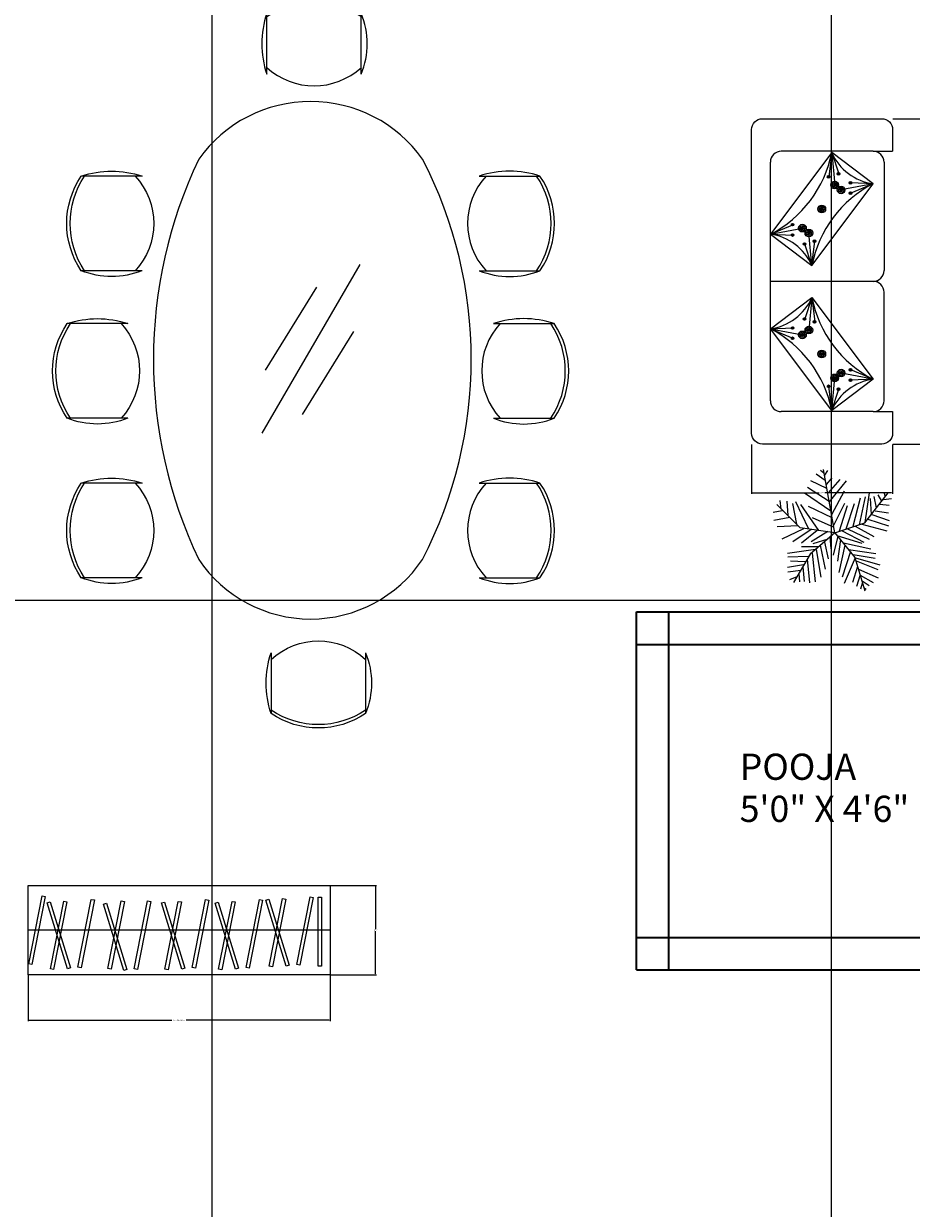
# Model space of a CAD drawing. Units: inches. Extents: x -61 to 1599, y -1316 to 257.
# Tile 196 of 204: x 1233 to 1396, y -279 to -61. Entities that reach past the tile are written whole.
import ezdxf

# ---------------------------------------------------------------- set-up
doc = ezdxf.new("R2010")
doc.units = ezdxf.units.IN
doc.header["$MEASUREMENT"] = 0
for name, color, linetype, lineweight in [('A-ANNO-DIMS', 2, 'Continuous', 18), ('A-AREA-IDEN', 1, 'Continuous', 18), ('A-FLOR-CASE', 8, 'Continuous', 18), ('FURNITURE', 83, 'Continuous', 18), ('WALLS', 4, 'Continuous', 35)]:
    doc.layers.add(name, color=color, linetype=linetype, lineweight=lineweight)
doc.layers.add('FUR', color=83, linetype='Continuous')
doc.styles.get("Standard").update_dxf_attribs({"font": 'arial.ttf'})
doc.dimstyles.get("Standard").update_dxf_attribs({"dimtxt": 0.18, "dimasz": 0.18, "dimexe": 0.18, "dimexo": 0.0625, "dimgap": 0.09, "dimtad": 0, "dimtih": 1, "dimtoh": 1, "dimdec": 0, "dimzin": 0, "dimdsep": 46, "dimlunit": 3, "dimtxsty": 'Standard', "dimcen": 0.09, "dimadec": 0, "dimazin": 0, "dimtfac": 1, "dimtdec": 0, "dimtofl": 0, "dimtmove": 0, "dimatfit": 3, "dimfxl": 1, "dimtolj": 1, "dimtzin": 0, "dimarcsym": 0})

# ---------------------------------------------------------------- blocks, each defined once
blk = doc.blocks.new('*U264')
for p, q in [((-10.186, 53.64), (-13.084, 55.962)), ((0, 0), (-10.5, 57)), ((-9.099, 51.782), (-6.563, 55.962)), ((-7.288, 39.707), (-21.778, 46.673)), ((-8.737, 47.138), (-17.069, 52.711)), ((-7.65, 43.423), (-2.578, 49.46)), ((-5.839, 35.992), (4.667, 48.067)), ((-5.114, 27.632), (10.463, 46.673)), ((-3.665, 19.273), (-27.574, 35.527)), ((-5.114, 28.097), (-24.676, 40.636)), ((-2.941, 16.486), (8.652, 37.85)), ((22.055, 7.198), (27.489, 32.277)), ((27, 9), (48, 36)), ((27.127, 9.056), (31.112, 35.992)), ((35.096, 32.741), (37.27, 22.524)), ((38.719, 34.134), (41.979, 28.561)), ((44.153, 36.456), (45.239, 32.741)), ((-31.5, 4.5), (-52.5, 25.5)), ((-48.585, 21.131), (-49.309, 29.026)), ((-43.513, 28.561), (-42.427, 15.558)), ((-38.442, 26.239), (-34.819, 7.663)), ((-35.544, 28.097), (-24.314, 3.947)), ((-14.533, 2.09), (-30.834, 25.31)), ((-24.314, 23.917), (-2.941, 13.7)), ((-1.129, 6.734), (9.014, 26.704)), ((3.942, 1.625), (11.187, 24.381)), ((10.101, 3.483), (17.708, 26.239)), ((16.259, 5.805), (23.142, 31.348)), ((31.836, 30.883), (32.561, 16.486)), ((40.53, 25.775), (48.862, 24.846)), ((43.791, 29.954), (51.036, 30.883)), ((-47.498, 19.737), (-55.83, 18.344)), ((-40.615, 13.7), (-55.105, 10.913)), ((-20.691, 13.7), (-1.129, 4.876)), ((29.662, 12.307), (48.137, 6.269)), ((33.285, 16.486), (48.862, 10.913)), ((36.183, 19.737), (48.137, 17.88)), ((-33.37, 6.269), (-52.207, 5.34)), ((-28.299, 3.483), (-47.86, -5.805)), ((-21.416, 3.018), (-38.079, -8.128)), ((0, 0), (-31.5, 4.5)), ((-15.982, 2.09), (-30.11, -9.521)), ((0, 0), (-22.5, -19.5)), ((-6.563, 1.161), (-21.416, -8.128)), ((0, 0), (27, 9)), ((0, 0), (18, -22.5)), ((6.478, 1.625), (26.04, -8.592)), ((11.187, 3.483), (30.749, -5.805)), ((18.07, 5.805), (35.096, -3.483)), ((24.229, 7.663), (46.688, 1.625)), ((-6.563, -5.805), (-19.967, -9.985)), ((-9.461, -8.592), (-6.201, -23.453)), ((-4.752, -3.483), (-3.665, -14.629)), ((2.493, -3.019), (-1.491, -20.202)), ((1.769, -2.555), (24.229, -9.521)), ((5.029, -6.27), (2.131, -25.775)), ((7.565, -9.056), (32.198, -14.629)), ((-17.431, -15.094), (-42.789, -18.809)), ((-22.5, -19.5), (-37.5, -45)), ((-15.257, -12.772), (-30.11, -12.772)), ((-20.691, -18.345), (-17.793, -44.352)), ((-17.069, -15.094), (-12.721, -40.172)), ((-13.446, -11.378), (-8.737, -32.741)), ((9.014, -11.378), (3.58, -35.992)), ((14.085, -16.951), (6.478, -40.172)), ((12.274, -15.094), (36.907, -18.809)), ((16.259, -19.738), (36.183, -22.989)), ((-28.299, -29.026), (-42.789, -31.348)), ((-24.314, -21.596), (-42.427, -22.06)), ((-26.849, -26.24), (-40.253, -25.775)), ((-29.023, -30.884), (-27.936, -43.887)), ((-25.038, -23.918), (-22.865, -45.281)), ((18.07, -22.524), (8.289, -45.745)), ((20.244, -30.419), (15.897, -44.816)), ((18, -22.5), (27, -52.5)), ((18.433, -22.524), (40.53, -29.026)), ((19.157, -25.311), (38.719, -33.206)), ((-30.834, -34.135), (-42.427, -35.528)), ((-34.457, -39.708), (-40.978, -42.494)), ((-32.646, -36.921), (-31.921, -44.352)), ((22.78, -37.85), (19.519, -48.532)), ((21.331, -32.741), (39.081, -40.636)), ((22.78, -38.314), (34.372, -44.816)), ((24.591, -45.745), (23.142, -50.854)), ((24.591, -43.423), (30.749, -47.603)), ((26.764, -49.925), (28.213, -50.854))]:
    blk.add_line(p, q)
blk = doc.blocks.new('DINING-TABLE-OVAL')
for p, q in [((20.06, 34.26), (38.12, 65.35)), ((20.69, 45.86), (30.12, 61.18)), ((27.51, 37.68), (36.94, 53.01))]:
    blk.add_line(p, q)
for centre, radius, start, end in [((28.99, 70.07), 25.36, 35.5172, 144.4828), ((85.79, 47.89), 85.79, 154.5151, 205.4849), ((-21.85, 47.89), 80.45, 332.689, 27.311), ((28.99, 24.89), 24.89, 213.9753, 326.0247)]:
    blk.add_arc(centre, radius, start, end)
blk = doc.blocks.new('DINING-CHAIR')
for p, q in [((0.9, 2.16), (0.9, 13.35)), ((18.35, 2.16), (18.35, 13.35))]:
    blk.add_line(p, q)
for centre, radius, start, end in [((9.63, 0.52), 15.52, 55.8098, 124.1902), ((9.63, -0.1), 15.52, 55.8098, 124.1902), ((17.78, 7.76), 17.78, 161.6455, 198.3545), ((4.51, 7.76), 14.92, 337.9646, 22.0354), ((9.63, 12.87), 12.87, 227.332, 312.668)]:
    blk.add_arc(centre, radius, start, end)
blk = doc.blocks.new('WARDROBE-HANGING-2')
blk.add_line((55.7, 8.23), (0, 8.23))
for points in [[(55.7, 16.46), (55.7, 0), (0, 0), (0, 16.46)], [(0.12, 2.03), (2.58, 14.54), (3.16, 14.43), (0.7, 1.92)], [(7.24, 1.1), (3.5, 13.29), (4.06, 13.46), (7.8, 1.28)], [(4.13, 1.08), (6.59, 13.59), (7.17, 13.48), (4.71, 0.97)], [(9.19, 1.4), (11.65, 13.91), (12.23, 13.8), (9.77, 1.29)], [(17.64, 0.82), (13.9, 13), (14.46, 13.18), (18.2, 0.99)], [(14.73, 1.14), (17.19, 13.65), (17.77, 13.54), (15.31, 1.03)], [(19.59, 1.12), (22.05, 13.62), (22.63, 13.51), (20.17, 1)], [(28.34, 1.05), (24.59, 13.24), (25.16, 13.41), (28.9, 1.22)], [(25.23, 1.03), (27.69, 13.54), (28.27, 13.43), (25.81, 0.92)], [(30.28, 1.35), (32.74, 13.86), (33.32, 13.75), (30.86, 1.24)], [(38.26, 1.05), (34.51, 13.23), (35.08, 13.41), (38.82, 1.22)], [(35.15, 1.03), (37.61, 13.54), (38.19, 13.42), (35.73, 0.92)], [(40.2, 1.35), (42.66, 13.86), (43.24, 13.74), (40.78, 1.23)], [(47.6, 1.58), (43.86, 13.76), (44.42, 13.94), (48.16, 1.75)], [(44.49, 1.56), (46.95, 14.07), (47.53, 13.95), (45.07, 1.45)], [(49.55, 1.88), (52.01, 14.39), (52.59, 14.27), (50.13, 1.77)], [(54.1, 14.33), (54.1, 1.58), (53.51, 1.58), (53.51, 14.33)]]:
    blk.add_lwpolyline(points, close=True)
blk = doc.blocks.new('*U160')
at = {"layer": 'FUR'}
blk.add_open_spline([(0, 0.08), (-0.03, 0.05), (-0.1, -0.02), (0.08, -0.02), (0.02, -0.06), (0, -0.08)], degree=3, knots=[0, 0, 0, 0, 0.0954578, 0.1898773, 0.2470677, 0.2470677, 0.2470677, 0.2470677], dxfattribs=at)
blk = doc.blocks.new('*U161')
at = {"layer": 'FUR', "transparency": 16777216}
for p, rotation in [((222.17, -79.98), 60), ((222.18, -80.06), 120), ((222.31, -79.97), 300), ((222.25, -80.09), 180), ((222.32, -80.05), 240)]:
    blk.add_blockref('*U160', p, dxfattribs=dict(at, rotation=rotation))
blk.add_blockref('*U160', (222.24, -79.93), dxfattribs=at)
blk = doc.blocks.new('*U172')
at = {"layer": 'FUR'}
blk.add_open_spline([(0, 0.08), (-0.03, 0.05), (-0.1, -0.02), (0.08, -0.02), (0.02, -0.06), (0, -0.08)], degree=3, knots=[0, 0, 0, 0, 0.0954578, 0.1898773, 0.2470677, 0.2470677, 0.2470677, 0.2470677], dxfattribs=at)
blk = doc.blocks.new('*U173')
at = {"layer": 'FUR', "transparency": 16777216}
for p, rotation in [((222.17, -79.98), 60), ((222.18, -80.06), 120), ((222.31, -79.97), 300), ((222.25, -80.09), 180), ((222.32, -80.05), 240)]:
    blk.add_blockref('*U172', p, dxfattribs=dict(at, rotation=rotation))
blk.add_blockref('*U172', (222.24, -79.93), dxfattribs=at)
blk = doc.blocks.new('*U186')
at = {"layer": 'FUR'}
blk.add_open_spline([(0, 0.08), (-0.03, 0.05), (-0.1, -0.02), (0.08, -0.02), (0.02, -0.06), (0, -0.08)], degree=3, knots=[0, 0, 0, 0, 0.0954578, 0.1898773, 0.2470677, 0.2470677, 0.2470677, 0.2470677], dxfattribs=at)
blk = doc.blocks.new('*U187')
at = {"layer": 'FUR', "transparency": 16777216}
for p, rotation in [((222.17, -79.98), 60), ((222.18, -80.06), 120), ((222.31, -79.97), 300), ((222.25, -80.09), 180), ((222.32, -80.05), 240)]:
    blk.add_blockref('*U186', p, dxfattribs=dict(at, rotation=rotation))
blk.add_blockref('*U186', (222.24, -79.93), dxfattribs=at)
blk = doc.blocks.new('*U198')
at = {"layer": 'FUR'}
blk.add_open_spline([(0, 0.08), (-0.03, 0.05), (-0.1, -0.02), (0.08, -0.02), (0.02, -0.06), (0, -0.08)], degree=3, knots=[0, 0, 0, 0, 0.0954578, 0.1898773, 0.2470677, 0.2470677, 0.2470677, 0.2470677], dxfattribs=at)
blk = doc.blocks.new('*U199')
at = {"layer": 'FUR', "transparency": 16777216}
for p, rotation in [((222.17, -79.98), 60), ((222.18, -80.06), 120), ((222.31, -79.97), 300), ((222.25, -80.09), 180), ((222.32, -80.05), 240)]:
    blk.add_blockref('*U198', p, dxfattribs=dict(at, rotation=rotation))
blk.add_blockref('*U198', (222.24, -79.93), dxfattribs=at)
blk = doc.blocks.new('*U184')
at = {"layer": 'FUR'}
blk.add_open_spline([(0.01, 0.24), (-0.09, 0.14), (-0.29, -0.05), (0.22, -0.05), (0.07, -0.19), (0.01, -0.24)], degree=3, knots=[0, 0, 0, 0, 0.2846533, 0.5662105, 0.736751, 0.736751, 0.736751, 0.736751], dxfattribs=at)
blk = doc.blocks.new('*U159')
at = {"layer": 'FUR', "transparency": 16777216}
for p, rotation in [((662.52, -238.49), 60), ((662.53, -238.73), 120), ((662.74, -238.83), 180), ((662.93, -238.46), 300), ((662.94, -238.7), 240)]:
    blk.add_blockref('*U184', p, dxfattribs=dict(at, rotation=rotation))
blk.add_blockref('*U184', (662.72, -238.36), dxfattribs=at)
blk = doc.blocks.new('*U210')
at = {"layer": 'FUR'}
blk.add_open_spline([(0.01, 0.24), (-0.09, 0.14), (-0.29, -0.05), (0.22, -0.05), (0.07, -0.19), (0.01, -0.24)], degree=3, knots=[0, 0, 0, 0, 0.2846533, 0.5662105, 0.736751, 0.736751, 0.736751, 0.736751], dxfattribs=at)
blk = doc.blocks.new('*U185')
at = {"layer": 'FUR', "transparency": 16777216}
for p, rotation in [((662.52, -238.49), 60), ((662.53, -238.73), 120), ((662.74, -238.83), 180), ((662.93, -238.46), 300), ((662.94, -238.7), 240)]:
    blk.add_blockref('*U210', p, dxfattribs=dict(at, rotation=rotation))
blk.add_blockref('*U210', (662.72, -238.36), dxfattribs=at)
blk = doc.blocks.new('*U174')
at = {"layer": 'FUR'}
blk.add_open_spline([(0, 0.08), (-0.03, 0.05), (-0.1, -0.02), (0.08, -0.02), (0.02, -0.06), (0, -0.08)], degree=3, knots=[0, 0, 0, 0, 0.0954578, 0.1898773, 0.2470677, 0.2470677, 0.2470677, 0.2470677], dxfattribs=at)
blk = doc.blocks.new('*U175')
at = {"layer": 'FUR', "transparency": 16777216}
for p, rotation in [((222.17, -79.98), 60), ((222.18, -80.06), 120), ((222.31, -79.97), 300), ((222.25, -80.09), 180), ((222.32, -80.05), 240)]:
    blk.add_blockref('*U174', p, dxfattribs=dict(at, rotation=rotation))
blk.add_blockref('*U174', (222.24, -79.93), dxfattribs=at)
blk = doc.blocks.new('*U200')
at = {"layer": 'FUR'}
blk.add_open_spline([(0, 0.08), (-0.03, 0.05), (-0.1, -0.02), (0.08, -0.02), (0.02, -0.06), (0, -0.08)], degree=3, knots=[0, 0, 0, 0, 0.0954578, 0.1898773, 0.2470677, 0.2470677, 0.2470677, 0.2470677], dxfattribs=at)
blk = doc.blocks.new('*U201')
at = {"layer": 'FUR', "transparency": 16777216}
for p, rotation in [((222.17, -79.98), 60), ((222.18, -80.06), 120), ((222.31, -79.97), 300), ((222.25, -80.09), 180), ((222.32, -80.05), 240)]:
    blk.add_blockref('*U200', p, dxfattribs=dict(at, rotation=rotation))
blk.add_blockref('*U200', (222.24, -79.93), dxfattribs=at)
blk = doc.blocks.new('*U168')
at = {"layer": 'FUR'}
blk.add_open_spline([(0.01, 0.24), (-0.09, 0.14), (-0.29, -0.05), (0.22, -0.05), (0.07, -0.19), (0.01, -0.24)], degree=3, knots=[0, 0, 0, 0, 0.2846533, 0.5662105, 0.736751, 0.736751, 0.736751, 0.736751], dxfattribs=at)
blk = doc.blocks.new('*U169')
at = {"layer": 'FUR', "transparency": 16777216}
for p, rotation in [((662.52, -238.49), 60), ((662.53, -238.73), 120), ((662.74, -238.83), 180), ((662.93, -238.46), 300), ((662.94, -238.7), 240)]:
    blk.add_blockref('*U168', p, dxfattribs=dict(at, rotation=rotation))
blk.add_blockref('*U168', (662.72, -238.36), dxfattribs=at)
blk = doc.blocks.new('*U194')
at = {"layer": 'FUR'}
blk.add_open_spline([(0.01, 0.24), (-0.09, 0.14), (-0.29, -0.05), (0.22, -0.05), (0.07, -0.19), (0.01, -0.24)], degree=3, knots=[0, 0, 0, 0, 0.2846533, 0.5662105, 0.736751, 0.736751, 0.736751, 0.736751], dxfattribs=at)
blk = doc.blocks.new('*U195')
at = {"layer": 'FUR', "transparency": 16777216}
for p, rotation in [((662.52, -238.49), 60), ((662.53, -238.73), 120), ((662.74, -238.83), 180), ((662.93, -238.46), 300), ((662.94, -238.7), 240)]:
    blk.add_blockref('*U194', p, dxfattribs=dict(at, rotation=rotation))
blk.add_blockref('*U194', (662.72, -238.36), dxfattribs=at)
blk = doc.blocks.new('*U176')
at = {"layer": 'FUR'}
blk.add_open_spline([(0, 0.08), (-0.03, 0.05), (-0.1, -0.02), (0.08, -0.02), (0.02, -0.06), (0, -0.08)], degree=3, knots=[0, 0, 0, 0, 0.0954578, 0.1898773, 0.2470677, 0.2470677, 0.2470677, 0.2470677], dxfattribs=at)
blk = doc.blocks.new('*U177')
at = {"layer": 'FUR', "transparency": 16777216}
for p, rotation in [((222.17, -79.98), 60), ((222.18, -80.06), 120), ((222.31, -79.97), 300), ((222.25, -80.09), 180), ((222.32, -80.05), 240)]:
    blk.add_blockref('*U176', p, dxfattribs=dict(at, rotation=rotation))
blk.add_blockref('*U176', (222.24, -79.93), dxfattribs=at)
blk = doc.blocks.new('*U202')
at = {"layer": 'FUR'}
blk.add_open_spline([(0, 0.08), (-0.03, 0.05), (-0.1, -0.02), (0.08, -0.02), (0.02, -0.06), (0, -0.08)], degree=3, knots=[0, 0, 0, 0, 0.0954578, 0.1898773, 0.2470677, 0.2470677, 0.2470677, 0.2470677], dxfattribs=at)
blk = doc.blocks.new('*U203')
at = {"layer": 'FUR', "transparency": 16777216}
for p, rotation in [((222.17, -79.98), 60), ((222.18, -80.06), 120), ((222.31, -79.97), 300), ((222.25, -80.09), 180), ((222.32, -80.05), 240)]:
    blk.add_blockref('*U202', p, dxfattribs=dict(at, rotation=rotation))
blk.add_blockref('*U202', (222.24, -79.93), dxfattribs=at)
blk = doc.blocks.new('*U170')
at = {"layer": 'FUR'}
blk.add_open_spline([(0.01, 0.24), (-0.09, 0.14), (-0.29, -0.05), (0.22, -0.05), (0.07, -0.19), (0.01, -0.24)], degree=3, knots=[0, 0, 0, 0, 0.2846533, 0.5662105, 0.736751, 0.736751, 0.736751, 0.736751], dxfattribs=at)
blk = doc.blocks.new('*U171')
at = {"layer": 'FUR', "transparency": 16777216}
for p, rotation in [((662.52, -238.49), 60), ((662.53, -238.73), 120), ((662.74, -238.83), 180), ((662.93, -238.46), 300), ((662.94, -238.7), 240)]:
    blk.add_blockref('*U170', p, dxfattribs=dict(at, rotation=rotation))
blk.add_blockref('*U170', (662.72, -238.36), dxfattribs=at)
blk = doc.blocks.new('*U196')
at = {"layer": 'FUR'}
blk.add_open_spline([(0.01, 0.24), (-0.09, 0.14), (-0.29, -0.05), (0.22, -0.05), (0.07, -0.19), (0.01, -0.24)], degree=3, knots=[0, 0, 0, 0, 0.2846533, 0.5662105, 0.736751, 0.736751, 0.736751, 0.736751], dxfattribs=at)
blk = doc.blocks.new('*U197')
at = {"layer": 'FUR', "transparency": 16777216}
for p, rotation in [((662.52, -238.49), 60), ((662.53, -238.73), 120), ((662.74, -238.83), 180), ((662.93, -238.46), 300), ((662.94, -238.7), 240)]:
    blk.add_blockref('*U196', p, dxfattribs=dict(at, rotation=rotation))
blk.add_blockref('*U196', (662.72, -238.36), dxfattribs=at)
blk = doc.blocks.new('*U164')
at = {"layer": 'FUR'}
blk.add_open_spline([(0, 0.08), (-0.03, 0.05), (-0.1, -0.02), (0.08, -0.02), (0.02, -0.06), (0, -0.08)], degree=3, knots=[0, 0, 0, 0, 0.0954578, 0.1898773, 0.2470677, 0.2470677, 0.2470677, 0.2470677], dxfattribs=at)
blk = doc.blocks.new('*U165')
at = {"layer": 'FUR', "transparency": 16777216}
for p, rotation in [((222.17, -79.98), 60), ((222.18, -80.06), 120), ((222.31, -79.97), 300), ((222.25, -80.09), 180), ((222.32, -80.05), 240)]:
    blk.add_blockref('*U164', p, dxfattribs=dict(at, rotation=rotation))
blk.add_blockref('*U164', (222.24, -79.93), dxfattribs=at)
blk = doc.blocks.new('*U190')
at = {"layer": 'FUR'}
blk.add_open_spline([(0, 0.08), (-0.03, 0.05), (-0.1, -0.02), (0.08, -0.02), (0.02, -0.06), (0, -0.08)], degree=3, knots=[0, 0, 0, 0, 0.0954578, 0.1898773, 0.2470677, 0.2470677, 0.2470677, 0.2470677], dxfattribs=at)
blk = doc.blocks.new('*U191')
at = {"layer": 'FUR', "transparency": 16777216}
for p, rotation in [((222.17, -79.98), 60), ((222.18, -80.06), 120), ((222.31, -79.97), 300), ((222.25, -80.09), 180), ((222.32, -80.05), 240)]:
    blk.add_blockref('*U190', p, dxfattribs=dict(at, rotation=rotation))
blk.add_blockref('*U190', (222.24, -79.93), dxfattribs=at)
blk = doc.blocks.new('*U183')
at = {"layer": 'FUR'}
blk.add_open_spline([(0.01, 0.24), (-0.09, 0.14), (-0.29, -0.05), (0.22, -0.05), (0.07, -0.19), (0.01, -0.24)], degree=3, knots=[0, 0, 0, 0, 0.2846533, 0.5662105, 0.736751, 0.736751, 0.736751, 0.736751], dxfattribs=at)
blk = doc.blocks.new('*U162')
at = {"layer": 'FUR', "transparency": 16777216}
for p, rotation in [((662.52, -238.49), 60), ((662.53, -238.73), 120), ((662.74, -238.83), 180), ((662.93, -238.46), 300), ((662.94, -238.7), 240)]:
    blk.add_blockref('*U183', p, dxfattribs=dict(at, rotation=rotation))
blk.add_blockref('*U183', (662.72, -238.36), dxfattribs=at)
blk = doc.blocks.new('*U209')
at = {"layer": 'FUR'}
blk.add_open_spline([(0.01, 0.24), (-0.09, 0.14), (-0.29, -0.05), (0.22, -0.05), (0.07, -0.19), (0.01, -0.24)], degree=3, knots=[0, 0, 0, 0, 0.2846533, 0.5662105, 0.736751, 0.736751, 0.736751, 0.736751], dxfattribs=at)
blk = doc.blocks.new('*U188')
at = {"layer": 'FUR', "transparency": 16777216}
for p, rotation in [((662.52, -238.49), 60), ((662.53, -238.73), 120), ((662.74, -238.83), 180), ((662.93, -238.46), 300), ((662.94, -238.7), 240)]:
    blk.add_blockref('*U209', p, dxfattribs=dict(at, rotation=rotation))
blk.add_blockref('*U209', (662.72, -238.36), dxfattribs=at)
blk = doc.blocks.new('*U182')
at = {"layer": 'FUR'}
blk.add_open_spline([(0, 0.08), (-0.03, 0.05), (-0.1, -0.02), (0.08, -0.02), (0.02, -0.06), (0, -0.08)], degree=3, knots=[0, 0, 0, 0, 0.0954578, 0.1898773, 0.2470677, 0.2470677, 0.2470677, 0.2470677], dxfattribs=at)
blk = doc.blocks.new('*U163')
at = {"layer": 'FUR', "transparency": 16777216}
for p, rotation in [((222.17, -79.98), 60), ((222.18, -80.06), 120), ((222.31, -79.97), 300), ((222.25, -80.09), 180), ((222.32, -80.05), 240)]:
    blk.add_blockref('*U182', p, dxfattribs=dict(at, rotation=rotation))
blk.add_blockref('*U182', (222.24, -79.93), dxfattribs=at)
blk = doc.blocks.new('*U208')
at = {"layer": 'FUR'}
blk.add_open_spline([(0, 0.08), (-0.03, 0.05), (-0.1, -0.02), (0.08, -0.02), (0.02, -0.06), (0, -0.08)], degree=3, knots=[0, 0, 0, 0, 0.0954578, 0.1898773, 0.2470677, 0.2470677, 0.2470677, 0.2470677], dxfattribs=at)
blk = doc.blocks.new('*U189')
at = {"layer": 'FUR', "transparency": 16777216}
for p, rotation in [((222.17, -79.98), 60), ((222.18, -80.06), 120), ((222.31, -79.97), 300), ((222.25, -80.09), 180), ((222.32, -80.05), 240)]:
    blk.add_blockref('*U208', p, dxfattribs=dict(at, rotation=rotation))
blk.add_blockref('*U208', (222.24, -79.93), dxfattribs=at)
blk = doc.blocks.new('*U166')
at = {"layer": 'FUR'}
blk.add_open_spline([(0.01, 0.24), (-0.09, 0.14), (-0.29, -0.05), (0.22, -0.05), (0.07, -0.19), (0.01, -0.24)], degree=3, knots=[0, 0, 0, 0, 0.2846533, 0.5662105, 0.736751, 0.736751, 0.736751, 0.736751], dxfattribs=at)
blk = doc.blocks.new('*U167')
at = {"layer": 'FUR', "transparency": 16777216}
for p, rotation in [((662.52, -238.49), 60), ((662.53, -238.73), 120), ((662.74, -238.83), 180), ((662.93, -238.46), 300), ((662.94, -238.7), 240)]:
    blk.add_blockref('*U166', p, dxfattribs=dict(at, rotation=rotation))
blk.add_blockref('*U166', (662.72, -238.36), dxfattribs=at)
blk = doc.blocks.new('*U192')
at = {"layer": 'FUR'}
blk.add_open_spline([(0.01, 0.24), (-0.09, 0.14), (-0.29, -0.05), (0.22, -0.05), (0.07, -0.19), (0.01, -0.24)], degree=3, knots=[0, 0, 0, 0, 0.2846533, 0.5662105, 0.736751, 0.736751, 0.736751, 0.736751], dxfattribs=at)
blk = doc.blocks.new('*U193')
at = {"layer": 'FUR', "transparency": 16777216}
for p, rotation in [((662.52, -238.49), 60), ((662.53, -238.73), 120), ((662.74, -238.83), 180), ((662.93, -238.46), 300), ((662.94, -238.7), 240)]:
    blk.add_blockref('*U192', p, dxfattribs=dict(at, rotation=rotation))
blk.add_blockref('*U192', (662.72, -238.36), dxfattribs=at)
blk = doc.blocks.new('*U178')
at = {"layer": 'FUR'}
blk.add_open_spline([(0, 0.08), (-0.03, 0.05), (-0.1, -0.02), (0.08, -0.02), (0.02, -0.06), (0, -0.08)], degree=3, knots=[0, 0, 0, 0, 0.0954578, 0.1898773, 0.2470677, 0.2470677, 0.2470677, 0.2470677], dxfattribs=at)
blk = doc.blocks.new('*U179')
at = {"layer": 'FUR', "transparency": 16777216}
for p, rotation in [((222.17, -79.98), 60), ((222.18, -80.06), 120), ((222.31, -79.97), 300), ((222.25, -80.09), 180), ((222.32, -80.05), 240)]:
    blk.add_blockref('*U178', p, dxfattribs=dict(at, rotation=rotation))
blk.add_blockref('*U178', (222.24, -79.93), dxfattribs=at)
blk = doc.blocks.new('*U180')
at = {"layer": 'FUR'}
blk.add_open_spline([(0, 0.08), (-0.03, 0.05), (-0.1, -0.02), (0.08, -0.02), (0.02, -0.06), (0, -0.08)], degree=3, knots=[0, 0, 0, 0, 0.0954578, 0.1898773, 0.2470677, 0.2470677, 0.2470677, 0.2470677], dxfattribs=at)
blk = doc.blocks.new('*U181')
at = {"layer": 'FUR', "transparency": 16777216}
for p, rotation in [((222.17, -79.98), 60), ((222.18, -80.06), 120), ((222.31, -79.97), 300), ((222.25, -80.09), 180), ((222.32, -80.05), 240)]:
    blk.add_blockref('*U180', p, dxfattribs=dict(at, rotation=rotation))
blk.add_blockref('*U180', (222.24, -79.93), dxfattribs=at)
blk = doc.blocks.new('*U204')
at = {"layer": 'FUR'}
blk.add_open_spline([(0, 0.08), (-0.03, 0.05), (-0.1, -0.02), (0.08, -0.02), (0.02, -0.06), (0, -0.08)], degree=3, knots=[0, 0, 0, 0, 0.0954578, 0.1898773, 0.2470677, 0.2470677, 0.2470677, 0.2470677], dxfattribs=at)
blk = doc.blocks.new('*U205')
at = {"layer": 'FUR', "transparency": 16777216}
for p, rotation in [((222.17, -79.98), 60), ((222.18, -80.06), 120), ((222.31, -79.97), 300), ((222.25, -80.09), 180), ((222.32, -80.05), 240)]:
    blk.add_blockref('*U204', p, dxfattribs=dict(at, rotation=rotation))
blk.add_blockref('*U204', (222.24, -79.93), dxfattribs=at)
blk = doc.blocks.new('*U206')
at = {"layer": 'FUR'}
blk.add_open_spline([(0, 0.08), (-0.03, 0.05), (-0.1, -0.02), (0.08, -0.02), (0.02, -0.06), (0, -0.08)], degree=3, knots=[0, 0, 0, 0, 0.0954578, 0.1898773, 0.2470677, 0.2470677, 0.2470677, 0.2470677], dxfattribs=at)
blk = doc.blocks.new('*U207')
at = {"layer": 'FUR', "transparency": 16777216}
for p, rotation in [((222.17, -79.98), 60), ((222.18, -80.06), 120), ((222.31, -79.97), 300), ((222.25, -80.09), 180), ((222.32, -80.05), 240)]:
    blk.add_blockref('*U206', p, dxfattribs=dict(at, rotation=rotation))
blk.add_blockref('*U206', (222.24, -79.93), dxfattribs=at)
blk = doc.blocks.new('SOFA-LOVESEAT')
for p, q in [((22.44, 54), (5.47, 54)), ((14.78, 53.75), (14.25, 49.29)), ((14.78, 53.75), (15.33, 47.76)), ((14.78, 53.75), (16.08, 49.82)), ((22.44, 54), (26, 54)), ((3.47, 8), (3.47, 52)), ((24.44, 52), (24.44, 32)), ((14.2, 49.3), (14.04, 49.3)), ((14.2, 49.3), (14.36, 49.3)), ((16.03, 49.84), (15.87, 49.84)), ((16.03, 49.84), (16.19, 49.84)), ((18.23, 48.19), (18.07, 48.19)), ((18.23, 48.19), (18.39, 48.19)), ((22.42, 48.01), (18.28, 48.17)), ((15.33, 47.76), (14.86, 47.76)), ((15.33, 47.76), (15.81, 47.76)), ((16.51, 46.87), (16.03, 46.87)), ((22.42, 48.01), (16.51, 46.87)), ((16.51, 46.87), (16.99, 46.87)), ((18.23, 46.28), (18.07, 46.28)), ((18.23, 46.28), (18.39, 46.28)), ((22.42, 48.01), (18.28, 46.26)), ((12.95, 43.35), (12.47, 43.35)), ((12.95, 43.35), (13.42, 43.35)), ((3.47, 38.69), (7.61, 40.44)), ((3.47, 38.69), (9.38, 39.83)), ((7.56, 40.46), (7.4, 40.46)), ((7.56, 40.46), (7.72, 40.46)), ((9.38, 39.83), (8.9, 39.83)), ((9.38, 39.83), (9.86, 39.83)), ((3.47, 38.69), (7.61, 38.53)), ((7.56, 38.55), (7.4, 38.55)), ((7.56, 38.55), (7.72, 38.55)), ((10.56, 38.94), (10.08, 38.94)), ((11.12, 32.95), (10.56, 38.94)), ((10.56, 38.94), (11.04, 38.94)), ((11.12, 32.95), (11.64, 37.41)), ((11.59, 37.43), (11.43, 37.43)), ((11.59, 37.43), (11.75, 37.43)), ((9.76, 36.9), (9.6, 36.9)), ((9.76, 36.9), (9.92, 36.9)), ((11.12, 32.95), (9.81, 36.88)), ((22.44, 30), (3.47, 30)), ((22.44, 30), (22.44, 30)), ((11.12, 27.03), (9.81, 23.09)), ((11.12, 27.03), (10.56, 21.03)), ((11.12, 27.03), (11.64, 22.56)), ((24.44, 8), (24.44, 28)), ((9.76, 23.07), (9.6, 23.07)), ((9.76, 23.07), (9.92, 23.07)), ((11.59, 22.54), (11.43, 22.54)), ((11.59, 22.54), (11.75, 22.54)), ((3.47, 21.29), (7.61, 21.44)), ((3.47, 21.29), (9.38, 20.15)), ((3.47, 21.29), (7.61, 19.54)), ((7.56, 21.42), (7.4, 21.42)), ((7.56, 21.42), (7.72, 21.42)), ((9.38, 20.15), (8.9, 20.15)), ((9.38, 20.15), (9.86, 20.15)), ((10.56, 21.03), (10.08, 21.03)), ((10.56, 21.03), (11.04, 21.03)), ((7.56, 19.52), (7.4, 19.52)), ((7.56, 19.52), (7.72, 19.52)), ((12.95, 16.62), (12.47, 16.62)), ((12.95, 16.62), (13.42, 16.62)), ((18.23, 13.69), (18.07, 13.69)), ((18.23, 13.69), (18.39, 13.69)), ((22.42, 11.96), (18.28, 13.71)), ((14.78, 6.22), (15.33, 12.22)), ((15.33, 12.22), (14.86, 12.22)), ((15.33, 12.22), (15.81, 12.22)), ((16.51, 13.1), (16.03, 13.1)), ((22.42, 11.96), (16.51, 13.1)), ((16.51, 13.1), (16.99, 13.1)), ((18.23, 11.79), (18.07, 11.79)), ((18.23, 11.79), (18.39, 11.79)), ((22.42, 11.96), (18.28, 11.81)), ((14.2, 10.67), (14.04, 10.67)), ((14.2, 10.67), (14.36, 10.67)), ((14.78, 6.22), (14.25, 10.69)), ((14.78, 6.22), (16.08, 10.16)), ((16.03, 10.14), (15.87, 10.14)), ((16.03, 10.14), (16.19, 10.14)), ((22.44, 6), (5.47, 6)), ((22.44, 6), (26, 6))]:
    blk.add_line(p, q)
blk.add_lwpolyline([(26, 6), (26, 2, -0.414214), (24, 0), (2, 0, -0.414214), (0, 2), (0, 58, -0.414213), (2, 60), (24, 60, -0.414214), (26, 58), (26, 54)], format="xyb")
for points in [[(11.12, 32.95), (22.42, 48.01), (14.78, 53.75), (3.47, 38.69)], [(11.12, 27.03), (22.42, 11.96), (14.78, 6.22), (3.47, 21.29)]]:
    blk.add_lwpolyline(points, close=True)
for centre, radius in [((14.2, 49.3), 0.238), ((14.2, 49.3), 0.16), ((15.33, 47.76), 0.71), ((15.33, 47.76), 0.476), ((16.03, 49.84), 0.238), ((16.03, 49.84), 0.16), ((18.23, 48.19), 0.238), ((18.23, 48.19), 0.16), ((16.51, 46.87), 0.71), ((16.51, 46.87), 0.476), ((18.23, 46.28), 0.238), ((18.23, 46.28), 0.16), ((12.95, 43.35), 0.71), ((12.95, 43.35), 0.476), ((7.56, 40.46), 0.238), ((7.56, 40.46), 0.16), ((9.38, 39.83), 0.71), ((9.38, 39.83), 0.476), ((10.56, 38.94), 0.71), ((10.56, 38.94), 0.476), ((7.56, 38.55), 0.238), ((7.56, 38.55), 0.16), ((9.76, 36.9), 0.238), ((11.59, 37.43), 0.238), ((11.59, 37.43), 0.16), ((9.76, 36.9), 0.16), ((9.76, 23.07), 0.238), ((9.76, 23.07), 0.16), ((11.59, 22.54), 0.238), ((11.59, 22.54), 0.16), ((7.56, 21.42), 0.238), ((7.56, 19.52), 0.238), ((7.56, 21.42), 0.16), ((7.56, 19.52), 0.16), ((9.38, 20.15), 0.71), ((9.38, 20.15), 0.476), ((10.56, 21.03), 0.71), ((10.56, 21.03), 0.476), ((12.95, 16.62), 0.71), ((12.95, 16.62), 0.476), ((16.51, 13.1), 0.71), ((16.51, 13.1), 0.476), ((18.23, 13.69), 0.238), ((18.23, 13.69), 0.16), ((15.33, 12.22), 0.71), ((15.33, 12.22), 0.476), ((18.23, 11.79), 0.238), ((18.23, 11.79), 0.16), ((14.2, 10.67), 0.238), ((14.2, 10.67), 0.16), ((16.03, 10.14), 0.238), ((16.03, 10.14), 0.16)]:
    blk.add_circle(centre, radius)
for centre, radius, start, end in [((5.47, 52), 2, 90, 180), ((-6.54, 57.97), 21.73, 297.4317, 348.7956), ((23.75, 57.74), 9.82, 203.9742, 262.253), ((22.44, 52), 2, 0, 90), ((32.43, 28.73), 21.73, 117.4317, 168.7956), ((2.15, 28.96), 9.82, 23.9742, 82.253), ((22.44, 32), 2, 270, 0), ((22.44, 28), 2, 0, 90), ((2.15, 31.01), 9.82, 277.747, 336.0258), ((32.43, 31.25), 21.73, 191.2044, 242.5684), ((-6.54, 2), 21.73, 11.2044, 62.5684), ((23.75, 2.23), 9.82, 97.747, 156.0258), ((5.47, 8), 2, 180, 270), ((22.44, 8), 2, 270, 0)]:
    blk.add_arc(centre, radius, start, end)
at = {"xscale": -1, "rotation": 90.00003000000098}
for name, p in [('*U191', (-65.81, 271.55)), ('*U188', (-223.26, 710.49)), ('*U189', (-63.98, 272.08)), ('*U205', (-61.78, 270.43)), ('*U193', (-222.08, 709.6)), ('*U207', (-61.78, 268.53)), ('*U197', (-225.65, 706.08)), ('*U187', (-72.45, 262.7)), ('*U185', (-229.21, 702.56)), ('*U195', (-228.03, 701.67)), ('*U199', (-72.45, 260.8)), ('*U203', (-68.43, 259.68)), ('*U201', (-70.25, 259.15))]:
    blk.add_blockref(name, p, dxfattribs=at)
at = {"rotation": 90}
for name, p in [('*U175', (-70.25, -199.17)), ('*U177', (-68.43, -199.7)), ('*U173', (-72.45, -200.82)), ('*U161', (-72.45, -202.73)), ('*U159', (-229.21, -642.58)), ('*U169', (-228.03, -641.7)), ('*U171', (-225.65, -646.11)), ('*U167', (-222.08, -649.63)), ('*U181', (-61.78, -208.55)), ('*U162', (-223.26, -650.51)), ('*U179', (-61.78, -210.46)), ('*U165', (-65.81, -211.58)), ('*U163', (-63.98, -212.11))]:
    blk.add_blockref(name, p, dxfattribs=at)
blk = doc.blocks.new('*D632')
at = {"layer": 'A-ANNO-DIMS', "color": 0, "lineweight": -2, "transparency": 16777216}
for p, q in [((1233.51, -236.29), (1233.51, -244.76)), ((1289.21, -236.29), (1289.21, -244.76)), ((1233.69, -244.58), (1260.05, -244.58)), ((1289.03, -244.58), (1262.67, -244.58))]:
    blk.add_line(p, q, dxfattribs=at)
at = {"layer": 'A-ANNO-DIMS', "color": 0, "transparency": 16777216}
for points in [[(1233.69, -244.55), (1233.69, -244.61), (1233.51, -244.58)], [(1289.03, -244.55), (1289.03, -244.61), (1289.21, -244.58)]]:
    blk.add_solid(points, dxfattribs=at)
at = {"layer": 'DEFPOINTS', "color": 0, "transparency": 16777216}
for p in [(1233.51, -236.23), (1289.21, -236.23), (1289.21, -244.58)]:
    blk.add_point(p, dxfattribs=at)
at = {"layer": 'A-ANNO-DIMS', "color": 0, "transparency": 16777216, "insert": (1261.36, -244.58), "char_height": 0.18, "attachment_point": 5}
blk.add_mtext('\\A1;WARDROBE 56 TYP.', dxfattribs=at)
blk = doc.blocks.new('*D633')
at = {"layer": 'A-ANNO-DIMS', "color": 0, "lineweight": -2, "transparency": 16777216}
for p, q in [((1289.27, -219.77), (1297.75, -219.77)), ((1297.57, -219.95), (1297.57, -227.81)), ((1297.57, -236.05), (1297.57, -228.18)), ((1289.27, -236.23), (1297.75, -236.23))]:
    blk.add_line(p, q, dxfattribs=at)
at = {"layer": 'A-ANNO-DIMS', "color": 0, "transparency": 16777216}
for points in [[(1297.54, -219.95), (1297.6, -219.95), (1297.57, -219.77)], [(1297.54, -236.05), (1297.6, -236.05), (1297.57, -236.23)]]:
    blk.add_solid(points, dxfattribs=at)
at = {"layer": 'DEFPOINTS', "color": 0, "transparency": 16777216}
for p in [(1289.21, -219.77), (1297.57, -219.77), (1289.21, -236.23)]:
    blk.add_point(p, dxfattribs=at)
at = {"layer": 'A-ANNO-DIMS', "color": 0, "transparency": 16777216, "insert": (1297.57, -228), "char_height": 0.18, "attachment_point": 5}
blk.add_mtext('\\A1;16 TYP.', dxfattribs=at)
blk = doc.blocks.new('*D636')
at = {"layer": 'A-ANNO-DIMS', "color": 0, "lineweight": -2, "transparency": 16777216}
for p, q in [((1393.01, -78.38), (1402.13, -78.38)), ((1401.95, -78.56), (1401.95, -108.2)), ((1401.95, -138.2), (1401.95, -108.57)), ((1393.01, -138.38), (1402.13, -138.38))]:
    blk.add_line(p, q, dxfattribs=at)
at = {"layer": 'A-ANNO-DIMS', "color": 0, "transparency": 16777216}
for points in [[(1401.92, -78.56), (1401.98, -78.56), (1401.95, -78.38)], [(1401.92, -138.2), (1401.98, -138.2), (1401.95, -138.38)]]:
    blk.add_solid(points, dxfattribs=at)
at = {"layer": 'DEFPOINTS', "color": 0, "transparency": 16777216}
for p in [(1392.95, -78.38), (1401.95, -78.38), (1392.95, -138.38)]:
    blk.add_point(p, dxfattribs=at)
at = {"layer": 'A-ANNO-DIMS', "color": 0, "transparency": 16777216, "insert": (1401.95, -108.38), "char_height": 0.18, "attachment_point": 5}
blk.add_mtext('\\A1;LOVESEAT 60 TYP.', dxfattribs=at)
blk = doc.blocks.new('*D637')
at = {"layer": 'A-ANNO-DIMS', "color": 0, "lineweight": -2, "transparency": 16777216}
for p, q in [((1366.95, -138.45), (1366.95, -147.56)), ((1392.95, -138.45), (1392.95, -147.56)), ((1367.13, -147.38), (1379.42, -147.38)), ((1392.77, -147.38), (1380.48, -147.38))]:
    blk.add_line(p, q, dxfattribs=at)
at = {"layer": 'A-ANNO-DIMS', "color": 0, "transparency": 16777216}
for points in [[(1367.13, -147.35), (1367.13, -147.41), (1366.95, -147.38)], [(1392.77, -147.35), (1392.77, -147.41), (1392.95, -147.38)]]:
    blk.add_solid(points, dxfattribs=at)
at = {"layer": 'DEFPOINTS', "color": 0, "transparency": 16777216}
for p in [(1366.95, -138.38), (1392.95, -138.38), (1392.95, -147.38)]:
    blk.add_point(p, dxfattribs=at)
at = {"layer": 'A-ANNO-DIMS', "color": 0, "transparency": 16777216, "insert": (1379.95, -147.38), "char_height": 0.18, "attachment_point": 5}
blk.add_mtext('\\A1;26 TYP.', dxfattribs=at)
blk = doc.blocks.new('*D698')
at = {"layer": 'A-ANNO-DIMS', "color": 0, "lineweight": -2, "transparency": 16777216}
for p, q in [((644.77, -167.17), (1598.48, -167.17)), ((1598.3, -167.35), (1598.3, -363.99)), ((1598.3, -560.99), (1598.3, -364.35)), ((644.77, -561.17), (1598.48, -561.17))]:
    blk.add_line(p, q, dxfattribs=at)
at = {"layer": 'A-ANNO-DIMS', "color": 0, "transparency": 16777216}
for points in [[(1598.27, -167.35), (1598.33, -167.35), (1598.3, -167.17)], [(1598.27, -560.99), (1598.33, -560.99), (1598.3, -561.17)]]:
    blk.add_solid(points, dxfattribs=at)
at = {"layer": 'DEFPOINTS', "color": 0, "transparency": 16777216}
for p in [(644.7, -167.17), (1598.3, -167.17), (644.7, -561.17)]:
    blk.add_point(p, dxfattribs=at)
at = {"layer": 'A-ANNO-DIMS', "color": 0, "transparency": 16777216, "insert": (1598.3, -364.17), "char_height": 0.18, "attachment_point": 5}
blk.add_mtext('\\A1;394', dxfattribs=at)
blk = doc.blocks.new('*D708')
at = {"layer": 'A-ANNO-DIMS', "color": 0, "lineweight": -2, "transparency": 16777216}
for p, q in [((1267.48, -588.11), (1267.48, 257.46)), ((1267.66, 257.28), (1324.14, 257.28)), ((1381.52, 257.28), (1325.05, 257.28)), ((1381.7, -588.11), (1381.7, 257.46))]:
    blk.add_line(p, q, dxfattribs=at)
at = {"layer": 'A-ANNO-DIMS', "color": 0, "transparency": 16777216}
for points in [[(1267.66, 257.31), (1267.66, 257.25), (1267.48, 257.28)], [(1381.52, 257.31), (1381.52, 257.25), (1381.7, 257.28)]]:
    blk.add_solid(points, dxfattribs=at)
at = {"layer": 'DEFPOINTS', "color": 0, "transparency": 16777216}
for p in [(1381.7, 257.28), (1267.48, -588.17), (1381.7, -588.17)]:
    blk.add_point(p, dxfattribs=at)
at = {"layer": 'A-ANNO-DIMS', "color": 0, "transparency": 16777216, "insert": (1324.59, 257.28), "char_height": 0.18, "attachment_point": 5}
blk.add_mtext('\\A1;114.22', dxfattribs=at)

msp = doc.modelspace()

# ---------------------------------------------------------------- linework, layer by layer
at = {"layer": 'WALLS'}
for p, q in [((1345.7028, -169.3229), (1381.7028, -169.3229)), ((1345.7028, -235.3229), (1345.7028, -169.3229)), ((1351.7028, -235.3229), (1351.7028, -169.3229)), ((1375.7028, -169.3229), (1522.7028, -169.3229)), ((1345.7028, -175.3229), (1351.7028, -175.3229)), ((1351.7028, -175.3229), (1411.7028, -175.3229)), ((1345.7028, -229.3229), (1522.7028, -229.3229)), ((1345.7028, -235.3229), (1522.7028, -235.3229))]:
    msp.add_line(p, q, dxfattribs=at)

# ---------------------------------------------------------------- block references
at = {"layer": 'A-FLOR-CASE'}
msp.add_blockref('WARDROBE-HANGING-2', (1233.5089, -236.2253), dxfattribs=at)
at = {"layer": 'FURNITURE'}
for name, p in [('DINING-CHAIR', (1276.622, -72.324)), ('DINING-TABLE-OVAL', (1256.634, -170.626)), ('SOFA-LOVESEAT', (1366.9518, -138.383))]:
    msp.add_blockref(name, p, dxfattribs=at)
at = {"layer": 'FURNITURE', "extrusion": (0, 0, -1), "zscale": -1}
for p, rotation in [((-1256.681, -88.0629), 269.9999999999987), ((-1254.0669, -115.2445), 269.9999999999985), ((-1256.681, -144.6698), 269.9999999999996), ((-1277.4166, -174.6778), 180)]:
    msp.add_blockref('DINING-CHAIR', p, dxfattribs=dict(at, rotation=rotation))
at = {"layer": 'FURNITURE'}
for p, rotation in [((1314.562, -88.0629), 269.9999999999997), ((1317.1761, -115.2445), 269.9999999999965), ((1314.562, -144.6698), 269.9999999999998)]:
    msp.add_blockref('DINING-CHAIR', p, dxfattribs=dict(at, rotation=rotation))
at = {"layer": 'FURNITURE', "xscale": 0.2045054661246738, "yscale": 0.2045054661246738, "zscale": 0.2045054661246738}
msp.add_blockref('*U264', (1382.3297, -154.712), dxfattribs=at)

# ---------------------------------------------------------------- texts
at = {"layer": 'A-AREA-IDEN'}
for s, height, p in [('POOJA', 4.8321, (1364.7531, -200.2805)), ('5\'0" X 4\'6"', 4.832098, (1364.7531, -208.0429))]:
    msp.add_text(s, height=height, dxfattribs=at).set_placement(p)

# ---------------------------------------------------------------- dimensions: what is measured, and where the dimension line sits
at = {"layer": 'A-ANNO-DIMS'}
dim = msp.add_linear_dim(base=(1381.7028, 257.2771), p1=(1267.4807, -588.169), p2=(1381.7028, -588.169), dimstyle='Standard', override={"dimdec": 2, "dimlfac": 1, "dimrnd": 0, "dimzin": 0, "dimdsep": 46, "dimlunit": 2}, dxfattribs=at)
dim.commit()
dim.dimension.update_dxf_attribs({"geometry": '*D708', "text_midpoint": (1324.5917, 257.2771)})
for base, p1, p2, text, picture, middle in [((1401.9522, -78.3832), (1392.9522, -138.3833), (1392.9522, -78.3832), 'LOVESEAT <> TYP.', '*D636', (1401.9522, -108.3832)), ((1297.5677, -219.7652), (1289.2121, -236.2252), (1289.2121, -219.7652), '<> TYP.', '*D633', (1297.5677, -227.9952))]:
    dim = msp.add_linear_dim(base=base, p1=p1, p2=p2, angle=90, text=text, dimstyle='Standard', override={"dimdec": 0, "dimlfac": 1, "dimrnd": 0, "dimzin": 0, "dimdsep": 46, "dimlunit": 2}, dxfattribs=at)
    dim.commit()
    dim.dimension.update_dxf_attribs({"geometry": picture, "text_midpoint": middle})
for base, p1, p2, text, picture, middle in [((1392.9522, -147.3833), (1366.9522, -138.3833), (1392.9522, -138.3833), '<> TYP.', '*D637', (1379.9522, -147.3833)), ((1289.2121, -244.5807), (1233.5087, -236.2252), (1289.2121, -236.2252), 'WARDROBE <> TYP.', '*D632', (1261.3604, -244.5807))]:
    dim = msp.add_linear_dim(base=base, p1=p1, p2=p2, text=text, dimstyle='Standard', override={"dimdec": 0, "dimlfac": 1, "dimrnd": 0, "dimzin": 0, "dimdsep": 46, "dimlunit": 2}, dxfattribs=at)
    dim.commit()
    dim.dimension.update_dxf_attribs({"geometry": picture, "text_midpoint": middle})
dim = msp.add_linear_dim(base=(1598.3028, -167.169), p1=(644.7028, -561.169), p2=(644.7028, -167.169), angle=90, dimstyle='Standard', override={"dimdec": 0, "dimlfac": 1, "dimrnd": 0, "dimzin": 0, "dimdsep": 46, "dimlunit": 2}, dxfattribs=at)
dim.commit()
dim.dimension.update_dxf_attribs({"geometry": '*D698', "text_midpoint": (1598.3028, -364.169)})

doc.saveas('drawing.dxf')
